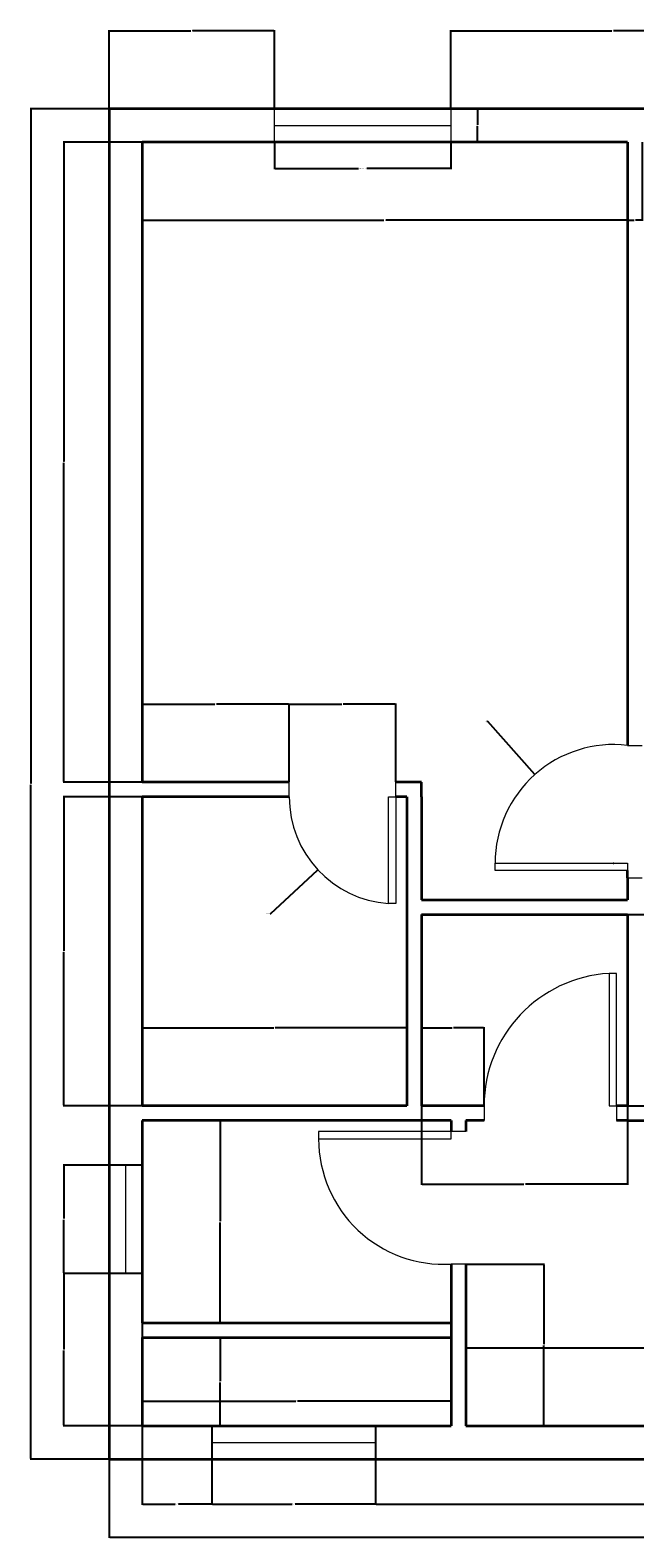
# Model space of a CAD drawing. Units: inches. Extents: x 2345 to 2781, y 2622 to 3032.
# Tile 1 of 3: x 2345 to 2509, y 2622 to 3032. Entities that reach past the tile are written whole.
import ezdxf

# ---------------------------------------------------------------- set-up
doc = ezdxf.new("R2010")
doc.units = ezdxf.units.IN
for name, color, linetype, lineweight in [('A-ANNO-DIMS', 2, 'Continuous', 18), ('A-DOOR', 3, 'Continuous', 18), ('A-GLAZ', 4, 'Continuous', 18), ('A-WALL', 7, 'Continuous', 35)]:
    doc.layers.add(name, color=color, linetype=linetype, lineweight=lineweight)
doc.styles.get("Standard").update_dxf_attribs({"font": 'arial.ttf'})
doc.dimstyles.get("Standard").update_dxf_attribs({"dimtxt": 0.18, "dimasz": 0.18, "dimexe": 0.18, "dimexo": 0.0625, "dimgap": 0.09, "dimtad": 0, "dimtih": 1, "dimtoh": 1, "dimdec": 4, "dimzin": 0, "dimdsep": 46, "dimtxsty": 'Standard', "dimcen": 0.09, "dimadec": 0, "dimazin": 0, "dimtfac": 1, "dimtdec": 4, "dimtofl": 0, "dimtmove": 0, "dimatfit": 3, "dimfxl": 1, "dimtolj": 1, "dimtzin": 0, "dimarcsym": 0})

# ---------------------------------------------------------------- blocks, each defined once
blk = doc.blocks.new('DOOR-36IN-SWING-A')
for p, q in [((36, 40), (34, 40)), ((34, 40), (34, 4)), ((36, 4), (36, 40)), ((0, 4), (0, 0)), ((34, 4), (36, 4)), ((36, 4), (36, 0))]:
    blk.add_line(p, q)
blk.add_arc((36.06, 4), 36.06, 93.2732, 180)
blk = doc.blocks.new('DOOR-36IN-SWING-B')
for p, q in [((0, 40), (0, 36)), ((36, 40), (36, 36)), ((0, 36), (0, 0)), ((2, 36), (0, 36)), ((2, 0), (2, 36)), ((0, 0), (2, 0))]:
    blk.add_line(p, q)
blk.add_arc((2, 34.06), 34.06, 270, 3.2732)
blk = doc.blocks.new('WIN-48IN')
for p, q in [((0, 0), (0, 9)), ((48, 0), (48, 9)), ((0, 4.5), (48, 4.5))]:
    blk.add_line(p, q)
blk = doc.blocks.new('*D8')
at = {"layer": 'A-ANNO-DIMS', "color": 0, "lineweight": -2, "transparency": 16777216}
for p, q in [((2411.27, 3001.74), (2411.27, 2994.42)), ((2459.27, 3001.74), (2459.27, 2994.42)), ((2411.45, 2994.6), (2434.15, 2994.6)), ((2459.09, 2994.6), (2436.39, 2994.6))]:
    blk.add_line(p, q, dxfattribs=at)
at = {"layer": 'A-ANNO-DIMS', "color": 0, "transparency": 16777216}
for points in [[(2411.45, 2994.63), (2411.45, 2994.57), (2411.27, 2994.6)], [(2459.09, 2994.63), (2459.09, 2994.57), (2459.27, 2994.6)]]:
    blk.add_solid(points, dxfattribs=at)
at = {"layer": 'Defpoints', "color": 0, "transparency": 16777216}
for p in [(2411.27, 3001.8), (2459.27, 3001.8), (2459.27, 2994.6)]:
    blk.add_point(p, dxfattribs=at)
at = {"layer": 'A-ANNO-DIMS', "color": 0, "transparency": 16777216, "insert": (2435.27, 2994.6), "char_height": 0.18, "attachment_point": 5}
blk.add_mtext('\\A1;WINDOW 48 TYP.', dxfattribs=at)
blk = doc.blocks.new('*D9')
at = {"layer": 'A-ANNO-DIMS', "color": 0, "lineweight": -2, "transparency": 16777216}
for p, q in [((2459.33, 3010.8), (2466.65, 3010.8)), ((2466.47, 3010.62), (2466.47, 3006.48)), ((2466.47, 3001.98), (2466.47, 3006.12)), ((2459.33, 3001.8), (2466.65, 3001.8))]:
    blk.add_line(p, q, dxfattribs=at)
at = {"layer": 'A-ANNO-DIMS', "color": 0, "transparency": 16777216}
for points in [[(2466.44, 3010.62), (2466.5, 3010.62), (2466.47, 3010.8)], [(2466.44, 3001.98), (2466.5, 3001.98), (2466.47, 3001.8)]]:
    blk.add_solid(points, dxfattribs=at)
at = {"layer": 'Defpoints', "color": 0, "transparency": 16777216}
for p in [(2459.27, 3010.8), (2466.47, 3010.8), (2459.27, 3001.8)]:
    blk.add_point(p, dxfattribs=at)
at = {"layer": 'A-ANNO-DIMS', "color": 0, "transparency": 16777216, "insert": (2466.47, 3006.3), "char_height": 0.18, "attachment_point": 5}
blk.add_mtext('\\A1;9 TYP.', dxfattribs=at)
blk = doc.blocks.new('*D10')
at = {"layer": 'A-ANNO-DIMS', "color": 0, "lineweight": -2, "transparency": 16777216}
for p, q in [((2366.27, 2643.74), (2366.27, 2622.37)), ((2768.27, 2643.74), (2768.27, 2622.37)), ((2366.45, 2622.55), (2566.98, 2622.55)), ((2768.09, 2622.55), (2567.56, 2622.55))]:
    blk.add_line(p, q, dxfattribs=at)
at = {"layer": 'A-ANNO-DIMS', "color": 0, "transparency": 16777216}
for points in [[(2366.45, 2622.58), (2366.45, 2622.52), (2366.27, 2622.55)], [(2768.09, 2622.58), (2768.09, 2622.52), (2768.27, 2622.55)]]:
    blk.add_solid(points, dxfattribs=at)
at = {"layer": 'Defpoints', "color": 0, "transparency": 16777216}
for p in [(2366.27, 2643.8), (2768.27, 2643.8), (2768.27, 2622.55)]:
    blk.add_point(p, dxfattribs=at)
at = {"layer": 'A-ANNO-DIMS', "color": 0, "transparency": 16777216, "insert": (2567.27, 2622.55), "char_height": 0.18, "attachment_point": 5}
blk.add_mtext('\\A1;402', dxfattribs=at)
blk = doc.blocks.new('*D11')
at = {"layer": 'A-ANNO-DIMS', "color": 0, "lineweight": -2, "transparency": 16777216}
for p, q in [((2366.21, 3010.8), (2344.84, 3010.8)), ((2345.02, 3010.62), (2345.02, 2827.48)), ((2345.02, 2643.98), (2345.02, 2827.12)), ((2366.21, 2643.8), (2344.84, 2643.8))]:
    blk.add_line(p, q, dxfattribs=at)
at = {"layer": 'A-ANNO-DIMS', "color": 0, "transparency": 16777216}
for points in [[(2344.99, 3010.62), (2345.05, 3010.62), (2345.02, 3010.8)], [(2344.99, 2643.98), (2345.05, 2643.98), (2345.02, 2643.8)]]:
    blk.add_solid(points, dxfattribs=at)
at = {"layer": 'Defpoints', "color": 0, "transparency": 16777216}
for p in [(2345.02, 3010.8), (2366.27, 3010.8), (2366.27, 2643.8)]:
    blk.add_point(p, dxfattribs=at)
at = {"layer": 'A-ANNO-DIMS', "color": 0, "transparency": 16777216, "insert": (2345.02, 2827.3), "char_height": 0.18, "attachment_point": 5}
blk.add_mtext('\\A1;367', dxfattribs=at)
blk = doc.blocks.new('*D12')
at = {"layer": 'A-ANNO-DIMS', "color": 0, "lineweight": -2, "transparency": 16777216}
for p, q in [((2366.27, 3010.87), (2366.27, 3032.23)), ((2366.45, 3032.05), (2388.55, 3032.05)), ((2411.09, 3032.05), (2389, 3032.05)), ((2411.27, 3010.87), (2411.27, 3032.23))]:
    blk.add_line(p, q, dxfattribs=at)
at = {"layer": 'A-ANNO-DIMS', "color": 0, "transparency": 16777216}
for points in [[(2366.45, 3032.08), (2366.45, 3032.02), (2366.27, 3032.05)], [(2411.09, 3032.08), (2411.09, 3032.02), (2411.27, 3032.05)]]:
    blk.add_solid(points, dxfattribs=at)
at = {"layer": 'Defpoints', "color": 0, "transparency": 16777216}
for p in [(2411.27, 3032.05), (2366.27, 3010.8), (2411.27, 3010.8)]:
    blk.add_point(p, dxfattribs=at)
at = {"layer": 'A-ANNO-DIMS', "color": 0, "transparency": 16777216, "insert": (2388.77, 3032.05), "char_height": 0.18, "attachment_point": 5}
blk.add_mtext('\\A1;45', dxfattribs=at)
blk = doc.blocks.new('*D13')
at = {"layer": 'A-ANNO-DIMS', "color": 0, "lineweight": -2, "transparency": 16777216}
for p, q in [((2459.27, 3010.87), (2459.27, 3032.23)), ((2459.45, 3032.05), (2503.05, 3032.05)), ((2547.09, 3032.05), (2503.49, 3032.05)), ((2547.27, 3010.87), (2547.27, 3032.23))]:
    blk.add_line(p, q, dxfattribs=at)
at = {"layer": 'A-ANNO-DIMS', "color": 0, "transparency": 16777216}
for points in [[(2459.45, 3032.08), (2459.45, 3032.02), (2459.27, 3032.05)], [(2547.09, 3032.08), (2547.09, 3032.02), (2547.27, 3032.05)]]:
    blk.add_solid(points, dxfattribs=at)
at = {"layer": 'Defpoints', "color": 0, "transparency": 16777216}
for p in [(2547.27, 3032.05), (2459.27, 3010.8), (2547.27, 3010.8)]:
    blk.add_point(p, dxfattribs=at)
at = {"layer": 'A-ANNO-DIMS', "color": 0, "transparency": 16777216, "insert": (2503.27, 3032.05), "char_height": 0.18, "attachment_point": 5}
blk.add_mtext('\\A1;88', dxfattribs=at)
blk = doc.blocks.new('*D15')
at = {"layer": 'A-ANNO-DIMS', "color": 0, "lineweight": -2, "transparency": 16777216}
for p, q in [((2375.27, 3001.74), (2375.27, 2980.37)), ((2507.27, 3001.74), (2507.27, 2980.37)), ((2375.45, 2980.55), (2440.99, 2980.55)), ((2507.09, 2980.55), (2441.55, 2980.55))]:
    blk.add_line(p, q, dxfattribs=at)
at = {"layer": 'A-ANNO-DIMS', "color": 0, "transparency": 16777216}
for points in [[(2375.45, 2980.58), (2375.45, 2980.52), (2375.27, 2980.55)], [(2507.09, 2980.58), (2507.09, 2980.52), (2507.27, 2980.55)]]:
    blk.add_solid(points, dxfattribs=at)
at = {"layer": 'Defpoints', "color": 0, "transparency": 16777216}
for p in [(2375.27, 3001.8), (2507.27, 3001.8), (2375.27, 2980.55)]:
    blk.add_point(p, dxfattribs=at)
at = {"layer": 'A-ANNO-DIMS', "color": 0, "transparency": 16777216, "insert": (2441.27, 2980.55), "char_height": 0.18, "attachment_point": 5}
blk.add_mtext('\\A1;132', dxfattribs=at)
blk = doc.blocks.new('*D16')
at = {"layer": 'A-ANNO-DIMS', "color": 0, "lineweight": -2, "transparency": 16777216}
for p, q in [((2507.27, 3001.74), (2507.27, 2980.37)), ((2511.27, 3001.74), (2511.27, 2980.37)), ((2507.45, 2980.55), (2509.12, 2980.55)), ((2511.09, 2980.55), (2509.42, 2980.55))]:
    blk.add_line(p, q, dxfattribs=at)
at = {"layer": 'A-ANNO-DIMS', "color": 0, "transparency": 16777216}
for points in [[(2507.45, 2980.58), (2507.45, 2980.52), (2507.27, 2980.55)], [(2511.09, 2980.58), (2511.09, 2980.52), (2511.27, 2980.55)]]:
    blk.add_solid(points, dxfattribs=at)
at = {"layer": 'Defpoints', "color": 0, "transparency": 16777216}
for p in [(2507.27, 3001.8), (2511.27, 3001.8), (2507.27, 2980.55)]:
    blk.add_point(p, dxfattribs=at)
at = {"layer": 'A-ANNO-DIMS', "color": 0, "transparency": 16777216, "insert": (2509.27, 2980.55), "char_height": 0.18, "attachment_point": 5}
blk.add_mtext('\\A1;4', dxfattribs=at)
blk = doc.blocks.new('*D24')
at = {"layer": 'A-ANNO-DIMS', "color": 0, "lineweight": -2, "transparency": 16777216}
for p, q in [((2375.21, 3001.8), (2353.84, 3001.8)), ((2354.02, 3001.62), (2354.02, 2914.98)), ((2354.02, 2827.98), (2354.02, 2914.62)), ((2375.21, 2827.8), (2353.84, 2827.8))]:
    blk.add_line(p, q, dxfattribs=at)
at = {"layer": 'A-ANNO-DIMS', "color": 0, "transparency": 16777216}
for points in [[(2353.99, 3001.62), (2354.05, 3001.62), (2354.02, 3001.8)], [(2353.99, 2827.98), (2354.05, 2827.98), (2354.02, 2827.8)]]:
    blk.add_solid(points, dxfattribs=at)
at = {"layer": 'Defpoints', "color": 0, "transparency": 16777216}
for p in [(2354.02, 3001.8), (2375.27, 3001.8), (2375.27, 2827.8)]:
    blk.add_point(p, dxfattribs=at)
at = {"layer": 'A-ANNO-DIMS', "color": 0, "transparency": 16777216, "insert": (2354.02, 2914.8), "char_height": 0.18, "attachment_point": 5}
blk.add_mtext('\\A1;174', dxfattribs=at)
blk = doc.blocks.new('*D26')
at = {"layer": 'A-ANNO-DIMS', "color": 0, "lineweight": -2, "transparency": 16777216}
for p, q in [((2375.27, 2827.87), (2375.27, 2849.23)), ((2375.45, 2849.05), (2395.05, 2849.05)), ((2415.09, 2849.05), (2395.49, 2849.05)), ((2415.27, 2827.87), (2415.27, 2849.23))]:
    blk.add_line(p, q, dxfattribs=at)
at = {"layer": 'A-ANNO-DIMS', "color": 0, "transparency": 16777216}
for points in [[(2375.45, 2849.08), (2375.45, 2849.02), (2375.27, 2849.05)], [(2415.09, 2849.08), (2415.09, 2849.02), (2415.27, 2849.05)]]:
    blk.add_solid(points, dxfattribs=at)
at = {"layer": 'Defpoints', "color": 0, "transparency": 16777216}
for p in [(2415.27, 2849.05), (2375.27, 2827.8), (2415.27, 2827.8)]:
    blk.add_point(p, dxfattribs=at)
at = {"layer": 'A-ANNO-DIMS', "color": 0, "transparency": 16777216, "insert": (2395.27, 2849.05), "char_height": 0.18, "attachment_point": 5}
blk.add_mtext('\\A1;40', dxfattribs=at)
blk = doc.blocks.new('*D27')
at = {"layer": 'A-ANNO-DIMS', "color": 0, "lineweight": -2, "transparency": 16777216}
for p, q in [((2415.27, 2827.87), (2415.27, 2849.23)), ((2415.45, 2849.05), (2429.55, 2849.05)), ((2444.09, 2849.05), (2429.99, 2849.05)), ((2444.27, 2827.87), (2444.27, 2849.23))]:
    blk.add_line(p, q, dxfattribs=at)
at = {"layer": 'A-ANNO-DIMS', "color": 0, "transparency": 16777216}
for points in [[(2415.45, 2849.08), (2415.45, 2849.02), (2415.27, 2849.05)], [(2444.09, 2849.08), (2444.09, 2849.02), (2444.27, 2849.05)]]:
    blk.add_solid(points, dxfattribs=at)
at = {"layer": 'Defpoints', "color": 0, "transparency": 16777216}
for p in [(2444.27, 2849.05), (2415.27, 2827.8), (2444.27, 2827.8)]:
    blk.add_point(p, dxfattribs=at)
at = {"layer": 'A-ANNO-DIMS', "color": 0, "transparency": 16777216, "insert": (2429.77, 2849.05), "char_height": 0.18, "attachment_point": 5}
blk.add_mtext('\\A1;29', dxfattribs=at)
blk = doc.blocks.new('*D32')
at = {"layer": 'A-ANNO-DIMS', "color": 0, "lineweight": -2, "transparency": 16777216}
for p, q in [((2375.27, 2739.87), (2375.27, 2761.23)), ((2375.45, 2761.05), (2411.05, 2761.05)), ((2447.09, 2761.05), (2411.49, 2761.05)), ((2447.27, 2739.87), (2447.27, 2761.23))]:
    blk.add_line(p, q, dxfattribs=at)
at = {"layer": 'A-ANNO-DIMS', "color": 0, "transparency": 16777216}
for points in [[(2375.45, 2761.08), (2375.45, 2761.02), (2375.27, 2761.05)], [(2447.09, 2761.08), (2447.09, 2761.02), (2447.27, 2761.05)]]:
    blk.add_solid(points, dxfattribs=at)
at = {"layer": 'Defpoints', "color": 0, "transparency": 16777216}
for p in [(2447.27, 2761.05), (2375.27, 2739.8), (2447.27, 2739.8)]:
    blk.add_point(p, dxfattribs=at)
at = {"layer": 'A-ANNO-DIMS', "color": 0, "transparency": 16777216, "insert": (2411.27, 2761.05), "char_height": 0.18, "attachment_point": 5}
blk.add_mtext('\\A1;72', dxfattribs=at)
blk = doc.blocks.new('*D33')
at = {"layer": 'A-ANNO-DIMS', "color": 0, "lineweight": -2, "transparency": 16777216}
for p, q in [((2375.21, 2823.8), (2353.84, 2823.8)), ((2354.02, 2823.62), (2354.02, 2781.98)), ((2354.02, 2739.98), (2354.02, 2781.62)), ((2375.21, 2739.8), (2353.84, 2739.8))]:
    blk.add_line(p, q, dxfattribs=at)
at = {"layer": 'A-ANNO-DIMS', "color": 0, "transparency": 16777216}
for points in [[(2353.99, 2823.62), (2354.05, 2823.62), (2354.02, 2823.8)], [(2353.99, 2739.98), (2354.05, 2739.98), (2354.02, 2739.8)]]:
    blk.add_solid(points, dxfattribs=at)
at = {"layer": 'Defpoints', "color": 0, "transparency": 16777216}
for p in [(2354.02, 2823.8), (2375.27, 2823.8), (2375.27, 2739.8)]:
    blk.add_point(p, dxfattribs=at)
at = {"layer": 'A-ANNO-DIMS', "color": 0, "transparency": 16777216, "insert": (2354.02, 2781.8), "char_height": 0.18, "attachment_point": 5}
blk.add_mtext('\\A1;84', dxfattribs=at)
blk = doc.blocks.new('*D34')
at = {"layer": 'A-ANNO-DIMS', "color": 0, "lineweight": -2, "transparency": 16777216}
for p, q in [((2507.33, 2791.8), (2528.7, 2791.8)), ((2528.52, 2791.62), (2528.52, 2765.98)), ((2528.52, 2739.98), (2528.52, 2765.62)), ((2507.33, 2739.8), (2528.7, 2739.8))]:
    blk.add_line(p, q, dxfattribs=at)
at = {"layer": 'A-ANNO-DIMS', "color": 0, "transparency": 16777216}
for points in [[(2528.49, 2791.62), (2528.55, 2791.62), (2528.52, 2791.8)], [(2528.49, 2739.98), (2528.55, 2739.98), (2528.52, 2739.8)]]:
    blk.add_solid(points, dxfattribs=at)
at = {"layer": 'Defpoints', "color": 0, "transparency": 16777216}
for p in [(2507.27, 2791.8), (2507.27, 2739.8), (2528.52, 2739.8)]:
    blk.add_point(p, dxfattribs=at)
at = {"layer": 'A-ANNO-DIMS', "color": 0, "transparency": 16777216, "insert": (2528.52, 2765.8), "char_height": 0.18, "attachment_point": 5}
blk.add_mtext('\\A1;52', dxfattribs=at)
blk = doc.blocks.new('*D35')
at = {"layer": 'A-ANNO-DIMS', "color": 0, "lineweight": -2, "transparency": 16777216}
for p, q in [((2451.27, 2739.74), (2451.27, 2718.37)), ((2507.27, 2739.74), (2507.27, 2718.37)), ((2451.45, 2718.55), (2479.05, 2718.55)), ((2507.09, 2718.55), (2479.49, 2718.55))]:
    blk.add_line(p, q, dxfattribs=at)
at = {"layer": 'A-ANNO-DIMS', "color": 0, "transparency": 16777216}
for points in [[(2451.45, 2718.58), (2451.45, 2718.52), (2451.27, 2718.55)], [(2507.09, 2718.58), (2507.09, 2718.52), (2507.27, 2718.55)]]:
    blk.add_solid(points, dxfattribs=at)
at = {"layer": 'Defpoints', "color": 0, "transparency": 16777216}
for p in [(2451.27, 2739.8), (2507.27, 2739.8), (2451.27, 2718.55)]:
    blk.add_point(p, dxfattribs=at)
at = {"layer": 'A-ANNO-DIMS', "color": 0, "transparency": 16777216, "insert": (2479.27, 2718.55), "char_height": 0.18, "attachment_point": 5}
blk.add_mtext('\\A1;56', dxfattribs=at)
blk = doc.blocks.new('*D37')
at = {"layer": 'A-ANNO-DIMS', "color": 0, "lineweight": -2, "transparency": 16777216}
for p, q in [((2451.27, 2739.87), (2451.27, 2761.23)), ((2451.45, 2761.05), (2459.56, 2761.05)), ((2468.09, 2761.05), (2459.98, 2761.05)), ((2468.27, 2739.87), (2468.27, 2761.23))]:
    blk.add_line(p, q, dxfattribs=at)
at = {"layer": 'A-ANNO-DIMS', "color": 0, "transparency": 16777216}
for points in [[(2451.45, 2761.08), (2451.45, 2761.02), (2451.27, 2761.05)], [(2468.09, 2761.08), (2468.09, 2761.02), (2468.27, 2761.05)]]:
    blk.add_solid(points, dxfattribs=at)
at = {"layer": 'Defpoints', "color": 0, "transparency": 16777216}
for p in [(2468.27, 2761.05), (2451.27, 2739.8), (2468.27, 2739.8)]:
    blk.add_point(p, dxfattribs=at)
at = {"layer": 'A-ANNO-DIMS', "color": 0, "transparency": 16777216, "insert": (2459.77, 2761.05), "char_height": 0.18, "attachment_point": 5}
blk.add_mtext('\\A1;17', dxfattribs=at)
blk = doc.blocks.new('*D49')
at = {"layer": 'A-ANNO-DIMS', "color": 0, "lineweight": -2, "transparency": 16777216}
for p, q in [((2375.27, 2680.74), (2375.27, 2659.37)), ((2459.27, 2680.74), (2459.27, 2659.37)), ((2375.45, 2659.55), (2417.05, 2659.55)), ((2459.09, 2659.55), (2417.49, 2659.55))]:
    blk.add_line(p, q, dxfattribs=at)
at = {"layer": 'A-ANNO-DIMS', "color": 0, "transparency": 16777216}
for points in [[(2375.45, 2659.58), (2375.45, 2659.52), (2375.27, 2659.55)], [(2459.09, 2659.58), (2459.09, 2659.52), (2459.27, 2659.55)]]:
    blk.add_solid(points, dxfattribs=at)
at = {"layer": 'Defpoints', "color": 0, "transparency": 16777216}
for p in [(2375.27, 2680.8), (2459.27, 2680.8), (2375.27, 2659.55)]:
    blk.add_point(p, dxfattribs=at)
at = {"layer": 'A-ANNO-DIMS', "color": 0, "transparency": 16777216, "insert": (2417.27, 2659.55), "char_height": 0.18, "attachment_point": 5}
blk.add_mtext('\\A1;84', dxfattribs=at)
blk = doc.blocks.new('*D50')
at = {"layer": 'A-ANNO-DIMS', "color": 0, "lineweight": -2, "transparency": 16777216}
for p, q in [((2375.33, 2676.8), (2396.7, 2676.8)), ((2396.52, 2676.62), (2396.52, 2664.98)), ((2396.52, 2652.98), (2396.52, 2664.62)), ((2375.33, 2652.8), (2396.7, 2652.8))]:
    blk.add_line(p, q, dxfattribs=at)
at = {"layer": 'A-ANNO-DIMS', "color": 0, "transparency": 16777216}
for points in [[(2396.49, 2676.62), (2396.55, 2676.62), (2396.52, 2676.8)], [(2396.49, 2652.98), (2396.55, 2652.98), (2396.52, 2652.8)]]:
    blk.add_solid(points, dxfattribs=at)
at = {"layer": 'Defpoints', "color": 0, "transparency": 16777216}
for p in [(2375.27, 2676.8), (2375.27, 2652.8), (2396.52, 2652.8)]:
    blk.add_point(p, dxfattribs=at)
at = {"layer": 'A-ANNO-DIMS', "color": 0, "transparency": 16777216, "insert": (2396.52, 2664.8), "char_height": 0.18, "attachment_point": 5}
blk.add_mtext('\\A1;24', dxfattribs=at)
blk = doc.blocks.new('*D51')
at = {"layer": 'A-ANNO-DIMS', "color": 0, "lineweight": -2, "transparency": 16777216}
for p, q in [((2375.33, 2735.8), (2396.7, 2735.8)), ((2396.52, 2735.62), (2396.52, 2708.48)), ((2396.52, 2680.98), (2396.52, 2708.12)), ((2375.33, 2680.8), (2396.7, 2680.8))]:
    blk.add_line(p, q, dxfattribs=at)
at = {"layer": 'A-ANNO-DIMS', "color": 0, "transparency": 16777216}
for points in [[(2396.49, 2735.62), (2396.55, 2735.62), (2396.52, 2735.8)], [(2396.49, 2680.98), (2396.55, 2680.98), (2396.52, 2680.8)]]:
    blk.add_solid(points, dxfattribs=at)
at = {"layer": 'Defpoints', "color": 0, "transparency": 16777216}
for p in [(2375.27, 2735.8), (2375.27, 2680.8), (2396.52, 2680.8)]:
    blk.add_point(p, dxfattribs=at)
at = {"layer": 'A-ANNO-DIMS', "color": 0, "transparency": 16777216, "insert": (2396.52, 2708.3), "char_height": 0.18, "attachment_point": 5}
blk.add_mtext('\\A1;55', dxfattribs=at)
blk = doc.blocks.new('*D52')
at = {"layer": 'A-ANNO-DIMS', "color": 0, "lineweight": -2, "transparency": 16777216}
for p, q in [((2463.27, 2652.87), (2463.27, 2674.23)), ((2463.45, 2674.05), (2537.99, 2674.05)), ((2613.09, 2674.05), (2538.55, 2674.05)), ((2613.27, 2652.87), (2613.27, 2674.23))]:
    blk.add_line(p, q, dxfattribs=at)
at = {"layer": 'A-ANNO-DIMS', "color": 0, "transparency": 16777216}
for points in [[(2463.45, 2674.08), (2463.45, 2674.02), (2463.27, 2674.05)], [(2613.09, 2674.08), (2613.09, 2674.02), (2613.27, 2674.05)]]:
    blk.add_solid(points, dxfattribs=at)
at = {"layer": 'Defpoints', "color": 0, "transparency": 16777216}
for p in [(2613.27, 2674.05), (2463.27, 2652.8), (2613.27, 2652.8)]:
    blk.add_point(p, dxfattribs=at)
at = {"layer": 'A-ANNO-DIMS', "color": 0, "transparency": 16777216, "insert": (2538.27, 2674.05), "char_height": 0.18, "attachment_point": 5}
blk.add_mtext('\\A1;150', dxfattribs=at)
blk = doc.blocks.new('*D55')
at = {"layer": 'A-ANNO-DIMS', "color": 0, "lineweight": -2, "transparency": 16777216}
for p, q in [((2463.334411, 2696.80295), (2484.701911, 2696.80295)), ((2484.521911, 2696.62295), (2484.521911, 2674.98295)), ((2484.521911, 2652.98295), (2484.521911, 2674.62295)), ((2463.334411, 2652.80295), (2484.701911, 2652.80295))]:
    blk.add_line(p, q, dxfattribs=at)
at = {"layer": 'A-ANNO-DIMS', "color": 0, "transparency": 16777216}
for points in [[(2484.491911, 2696.62295), (2484.551911, 2696.62295), (2484.521911, 2696.80295)], [(2484.491911, 2652.98295), (2484.551911, 2652.98295), (2484.521911, 2652.80295)]]:
    blk.add_solid(points, dxfattribs=at)
at = {"layer": 'Defpoints', "color": 0, "transparency": 16777216}
for p in [(2463.271911, 2696.80295), (2463.271911, 2652.80295), (2484.521911, 2652.80295)]:
    blk.add_point(p, dxfattribs=at)
at = {"layer": 'A-ANNO-DIMS', "color": 0, "transparency": 16777216, "insert": (2484.521911, 2674.80295), "char_height": 0.18, "attachment_point": 5}
blk.add_mtext('\\A1;44', dxfattribs=at)
blk = doc.blocks.new('*D57')
at = {"layer": 'A-ANNO-DIMS', "color": 0, "lineweight": -2, "transparency": 16777216}
for p, q in [((2375.27, 2652.74), (2375.27, 2631.37)), ((2394.21, 2652.74), (2394.21, 2631.37)), ((2375.45, 2631.55), (2384.28, 2631.55)), ((2394.03, 2631.55), (2385.19, 2631.55))]:
    blk.add_line(p, q, dxfattribs=at)
at = {"layer": 'A-ANNO-DIMS', "color": 0, "transparency": 16777216}
for points in [[(2375.45, 2631.58), (2375.45, 2631.52), (2375.27, 2631.55)], [(2394.03, 2631.58), (2394.03, 2631.52), (2394.21, 2631.55)]]:
    blk.add_solid(points, dxfattribs=at)
at = {"layer": 'Defpoints', "color": 0, "transparency": 16777216}
for p in [(2375.27, 2652.8), (2394.21, 2652.8), (2375.27, 2631.55)]:
    blk.add_point(p, dxfattribs=at)
at = {"layer": 'A-ANNO-DIMS', "color": 0, "transparency": 16777216, "insert": (2384.74, 2631.55), "char_height": 0.18, "attachment_point": 5}
blk.add_mtext('\\A1;18.934', dxfattribs=at)
blk = doc.blocks.new('*D58')
at = {"layer": 'A-ANNO-DIMS', "color": 0, "lineweight": -2, "transparency": 16777216}
for p, q in [((2394.21, 2652.74), (2394.21, 2631.37)), ((2438.77, 2652.74), (2438.77, 2631.37)), ((2394.39, 2631.55), (2416.09, 2631.55)), ((2438.59, 2631.55), (2416.88, 2631.55))]:
    blk.add_line(p, q, dxfattribs=at)
at = {"layer": 'A-ANNO-DIMS', "color": 0, "transparency": 16777216}
for points in [[(2394.39, 2631.58), (2394.39, 2631.52), (2394.21, 2631.55)], [(2438.59, 2631.58), (2438.59, 2631.52), (2438.77, 2631.55)]]:
    blk.add_solid(points, dxfattribs=at)
at = {"layer": 'Defpoints', "color": 0, "transparency": 16777216}
for p in [(2394.21, 2652.8), (2438.77, 2652.8), (2394.21, 2631.55)]:
    blk.add_point(p, dxfattribs=at)
at = {"layer": 'A-ANNO-DIMS', "color": 0, "transparency": 16777216, "insert": (2416.49, 2631.55), "char_height": 0.18, "attachment_point": 5}
blk.add_mtext('\\A1;44.56', dxfattribs=at)
blk = doc.blocks.new('*D59')
at = {"layer": 'A-ANNO-DIMS', "color": 0, "lineweight": -2, "transparency": 16777216}
for p, q in [((2438.77, 2652.74), (2438.77, 2631.37)), ((2637.97, 2652.74), (2637.97, 2631.37)), ((2438.95, 2631.55), (2537.98, 2631.55)), ((2637.79, 2631.55), (2538.75, 2631.55))]:
    blk.add_line(p, q, dxfattribs=at)
at = {"layer": 'A-ANNO-DIMS', "color": 0, "transparency": 16777216}
for points in [[(2438.95, 2631.58), (2438.95, 2631.52), (2438.77, 2631.55)], [(2637.79, 2631.58), (2637.79, 2631.52), (2637.97, 2631.55)]]:
    blk.add_solid(points, dxfattribs=at)
at = {"layer": 'Defpoints', "color": 0, "transparency": 16777216}
for p in [(2438.77, 2652.8), (2637.97, 2652.8), (2438.77, 2631.55)]:
    blk.add_point(p, dxfattribs=at)
at = {"layer": 'A-ANNO-DIMS', "color": 0, "transparency": 16777216, "insert": (2538.37, 2631.55), "char_height": 0.18, "attachment_point": 5}
blk.add_mtext('\\A1;199.2', dxfattribs=at)
blk = doc.blocks.new('*D63')
at = {"layer": 'A-ANNO-DIMS', "color": 0, "lineweight": -2, "transparency": 16777216}
for p, q in [((2375.21, 2723.72), (2353.84, 2723.72)), ((2354.02, 2723.54), (2354.02, 2709.16)), ((2354.02, 2694.41), (2354.02, 2708.79)), ((2375.21, 2694.23), (2353.84, 2694.23))]:
    blk.add_line(p, q, dxfattribs=at)
at = {"layer": 'A-ANNO-DIMS', "color": 0, "transparency": 16777216}
for points in [[(2353.99, 2723.54), (2354.05, 2723.54), (2354.02, 2723.72)], [(2353.99, 2694.41), (2354.05, 2694.41), (2354.02, 2694.23)]]:
    blk.add_solid(points, dxfattribs=at)
at = {"layer": 'Defpoints', "color": 0, "transparency": 16777216}
for p in [(2354.02, 2723.72), (2375.27, 2723.72), (2375.27, 2694.23)]:
    blk.add_point(p, dxfattribs=at)
at = {"layer": 'A-ANNO-DIMS', "color": 0, "transparency": 16777216, "insert": (2354.02, 2708.97), "char_height": 0.18, "attachment_point": 5}
blk.add_mtext('\\A1;29.48', dxfattribs=at)
blk = doc.blocks.new('*D64')
at = {"layer": 'A-ANNO-DIMS', "color": 0, "lineweight": -2, "transparency": 16777216}
for p, q in [((2375.21, 2694.23), (2353.84, 2694.23)), ((2354.02, 2694.05), (2354.02, 2673.7)), ((2354.02, 2652.98), (2354.02, 2673.34)), ((2375.21, 2652.8), (2353.84, 2652.8))]:
    blk.add_line(p, q, dxfattribs=at)
at = {"layer": 'A-ANNO-DIMS', "color": 0, "transparency": 16777216}
for points in [[(2353.99, 2694.05), (2354.05, 2694.05), (2354.02, 2694.23)], [(2353.99, 2652.98), (2354.05, 2652.98), (2354.02, 2652.8)]]:
    blk.add_solid(points, dxfattribs=at)
at = {"layer": 'Defpoints', "color": 0, "transparency": 16777216}
for p in [(2354.02, 2694.23), (2375.27, 2694.23), (2375.27, 2652.8)]:
    blk.add_point(p, dxfattribs=at)
at = {"layer": 'A-ANNO-DIMS', "color": 0, "transparency": 16777216, "insert": (2354.02, 2673.52), "char_height": 0.18, "attachment_point": 5}
blk.add_mtext('\\A1;41.43', dxfattribs=at)
blk = doc.blocks.new('*D67')
at = {"layer": 'A-ANNO-DIMS', "color": 0, "lineweight": -2, "transparency": 16777216}
for p, q in [((2469.06, 2844.34), (2469.24, 2844.34)), ((2469.24, 2844.34), (2481.97, 2830.02)), ((2503.4, 2805.8), (2503.58, 2805.8)), ((2503.49, 2805.71), (2503.49, 2805.89))]:
    blk.add_line(p, q, dxfattribs=at)
at = {"layer": 'A-ANNO-DIMS', "color": 0, "transparency": 16777216}
blk.add_solid([(2481.99, 2830.04), (2481.94, 2830), (2482.09, 2829.89)], dxfattribs=at)
at = {"layer": 'Defpoints', "color": 0, "transparency": 16777216}
for p in [(2482.09, 2829.89), (2503.49, 2805.8)]:
    blk.add_point(p, dxfattribs=at)
at = {"layer": 'A-ANNO-DIMS', "color": 0, "transparency": 16777216, "insert": (2468.58, 2844.34), "char_height": 0.18, "attachment_point": 5}
blk.add_mtext('\\A1;R32.22', dxfattribs=at)
blk = doc.blocks.new('*D68')
at = {"layer": 'A-ANNO-DIMS', "color": 0, "lineweight": -2, "transparency": 16777216}
for p, q in [((2444.26, 2823.8), (2444.44, 2823.8)), ((2444.35, 2823.71), (2444.35, 2823.89)), ((2410.3, 2792.1), (2422.94, 2803.87)), ((2410.12, 2792.1), (2410.3, 2792.1))]:
    blk.add_line(p, q, dxfattribs=at)
at = {"layer": 'A-ANNO-DIMS', "color": 0, "transparency": 16777216}
blk.add_solid([(2422.91, 2803.89), (2422.96, 2803.85), (2423.07, 2803.99)], dxfattribs=at)
at = {"layer": 'Defpoints', "color": 0, "transparency": 16777216}
for p in [(2444.35, 2823.8), (2423.07, 2803.99)]:
    blk.add_point(p, dxfattribs=at)
at = {"layer": 'A-ANNO-DIMS', "color": 0, "transparency": 16777216, "insert": (2409.57, 2792.1), "char_height": 0.18, "attachment_point": 5}
blk.add_mtext('\\A1;R29.074', dxfattribs=at)

msp = doc.modelspace()

# ---------------------------------------------------------------- linework, layer by layer
at = {"layer": 'A-DOOR'}
for p, q in [((2507.2719, 2837.803), (2511.2719, 2837.803)), ((2415.2719, 2823.8029), (2415.2719, 2827.8029)), ((2444.2719, 2823.8029), (2444.2719, 2827.8029)), ((2442.2719, 2794.803), (2442.2719, 2823.8029)), ((2442.2719, 2823.8029), (2445.7719, 2823.8029)), ((2444.2719, 2823.8029), (2444.2719, 2794.803)), ((2471.2719, 2803.803), (2471.2719, 2805.8029)), ((2471.2719, 2805.8029), (2507.2719, 2805.8029)), ((2507.2719, 2803.803), (2471.2719, 2803.803)), ((2507.2719, 2805.8029), (2507.2719, 2803.803)), ((2507.2719, 2801.803), (2511.2719, 2801.803)), ((2444.2719, 2794.803), (2442.2719, 2794.803))]:
    msp.add_line(p, q, dxfattribs=at)
for centre, radius, start, end in [((2503.4941, 2805.8029), 32.2222, 83.267079, 180), ((2444.346, 2823.8029), 29.0741, 180, 265.909183)]:
    msp.add_arc(centre, radius, start, end, dxfattribs=at)
at = {"layer": 'A-GLAZ'}
for p, q in [((2375.2719, 2723.7151), (2366.2719, 2723.7151)), ((2370.7719, 2723.7151), (2370.7719, 2694.2347)), ((2375.2719, 2694.2347), (2366.2719, 2694.2347)), ((2394.2063, 2652.8029), (2394.2063, 2643.8029)), ((2438.7687, 2652.8029), (2438.7687, 2643.8029)), ((2394.2063, 2648.303), (2438.7687, 2648.303))]:
    msp.add_line(p, q, dxfattribs=at)
at = {"layer": 'A-WALL'}
for p, q in [((2768.2719, 3010.8029), (2366.2719, 3010.8029)), ((2366.2719, 3010.8029), (2366.2719, 2643.8029)), ((2375.2719, 3001.8029), (2375.2719, 2827.8029)), ((2507.2719, 3001.8029), (2375.2719, 3001.8029)), ((2507.2719, 3001.8029), (2507.2719, 2837.803)), ((2415.2719, 2827.8029), (2375.2719, 2827.8029)), ((2451.2719, 2827.8029), (2444.2719, 2827.8029)), ((2451.2719, 2823.8029), (2451.2719, 2827.8029)), ((2375.2719, 2823.8029), (2375.2719, 2739.8029)), ((2415.2719, 2823.8029), (2375.2719, 2823.8029)), ((2447.2719, 2823.8029), (2444.2719, 2823.8029)), ((2447.2719, 2823.8029), (2447.2719, 2739.8029)), ((2451.2719, 2823.8029), (2451.2719, 2795.803)), ((2451.2719, 2823.8029), (2451.2719, 2795.803)), ((2507.2719, 2801.803), (2507.2719, 2803.803)), ((2507.2719, 2801.803), (2507.2719, 2795.803)), ((2451.2719, 2795.803), (2507.2719, 2795.803)), ((2451.2719, 2791.8029), (2507.2719, 2791.8029)), ((2451.2719, 2791.8029), (2451.2719, 2779.803)), ((2451.2719, 2791.8029), (2451.2719, 2779.803)), ((2507.2719, 2791.8029), (2507.2719, 2779.803)), ((2451.2719, 2779.803), (2451.2719, 2775.0862)), ((2507.2719, 2779.803), (2507.2719, 2774.511)), ((2451.2719, 2775.803), (2451.2719, 2739.8029)), ((2451.2719, 2775.803), (2451.2719, 2739.8029)), ((2507.2719, 2775.803), (2507.2719, 2739.8029)), ((2447.2719, 2739.8029), (2375.2719, 2739.8029)), ((2468.2719, 2739.8029), (2451.2719, 2739.8029)), ((2507.2719, 2739.8029), (2504.2719, 2739.8029)), ((2375.2719, 2735.8029), (2375.2719, 2680.8029)), ((2459.2719, 2735.8029), (2375.2719, 2735.8029)), ((2459.2719, 2735.8029), (2459.2719, 2732.803)), ((2468.2719, 2735.8029), (2463.2719, 2735.8029)), ((2463.2719, 2735.8029), (2463.2719, 2732.803)), ((2507.2719, 2735.8029), (2504.2719, 2735.8029)), ((2507.2719, 2735.8029), (2511.7641, 2735.8029)), ((2459.2719, 2696.8029), (2459.2719, 2652.8029)), ((2463.2719, 2696.8029), (2463.2719, 2652.8029)), ((2375.2719, 2680.8029), (2459.2719, 2680.8029)), ((2375.2719, 2676.8029), (2459.2719, 2676.8029)), ((2375.2719, 2676.8029), (2375.2719, 2652.8029)), ((2375.2719, 2652.8029), (2459.2719, 2652.8029)), ((2463.2719, 2652.8029), (2507.2719, 2652.8029)), ((2507.2719, 2652.8029), (2513.846, 2652.8029)), ((2366.2719, 2643.8029), (2768.2719, 2643.8029))]:
    msp.add_line(p, q, dxfattribs=at)

# ---------------------------------------------------------------- block references
at = {"layer": 'A-DOOR'}
msp.add_blockref('DOOR-36IN-SWING-A', (2468.272, 2735.803), dxfattribs=at)
at = {"layer": 'A-DOOR', "rotation": 270.0000000000041}
msp.add_blockref('DOOR-36IN-SWING-B', (2423.272, 2732.8029), dxfattribs=at)
at = {"layer": 'A-GLAZ'}
msp.add_blockref('WIN-48IN', (2411.272, 3001.803), dxfattribs=at)

# ---------------------------------------------------------------- dimensions: what is measured, and where the dimension line sits
at = {"layer": 'A-ANNO-DIMS'}
for base, p1, p2, picture, middle in [((2411.2719, 3032.0529), (2366.2719, 3010.8029), (2411.2719, 3010.8029), '*D12', (2388.7719, 3032.0529)), ((2547.2719, 3032.0529), (2459.2719, 3010.8029), (2547.2719, 3010.8029), '*D13', (2503.2719, 3032.0529)), ((2415.2719, 2849.0529), (2375.2719, 2827.8029), (2415.2719, 2827.8029), '*D26', (2395.2719, 2849.0529)), ((2444.2719, 2849.0529), (2415.2719, 2827.8029), (2444.2719, 2827.8029), '*D27', (2429.7719, 2849.0529)), ((2447.2719, 2761.0529), (2375.2719, 2739.8029), (2447.2719, 2739.8029), '*D32', (2411.2719, 2761.0529)), ((2468.2719, 2761.0529), (2451.2719, 2739.8029), (2468.2719, 2739.8029), '*D37', (2459.7719, 2761.0529)), ((2768.2719, 2622.5529), (2366.2719, 2643.8029), (2768.2719, 2643.8029), '*D10', (2567.2719, 2622.5529))]:
    dim = msp.add_linear_dim(base=base, p1=p1, p2=p2, dimstyle='Standard', override={"dimdec": 0, "dimlfac": 1, "dimrnd": 0, "dimzin": 0, "dimdsep": 46, "dimlunit": 2}, dxfattribs=at)
    dim.commit()
    dim.dimension.update_dxf_attribs({"geometry": picture, "text_midpoint": middle})
for base, p1, p2, angle, override, picture, middle in [((2345.0219, 3010.8029), (2366.2719, 2643.8029), (2366.2719, 3010.8029), 90, {"dimdec": 0, "dimlfac": 1, "dimrnd": 0, "dimzin": 0, "dimdsep": 46, "dimlunit": 2}, '*D11', (2345.0219, 2827.3029)), ((2354.0219, 3001.8029), (2375.2719, 2827.8029), (2375.2719, 3001.8029), 90, {"dimdec": 0, "dimlfac": 1, "dimrnd": 0, "dimzin": 0, "dimdsep": 46, "dimlunit": 2}, '*D24', (2354.0219, 2914.8029)), ((2375.2719, 2980.5529), (2507.2719, 3001.8029), (2375.2719, 3001.8029), 180, {"dimdec": 0, "dimlfac": 1, "dimrnd": 0, "dimzin": 0, "dimdsep": 46, "dimlunit": 2}, '*D15', (2441.2719, 2980.5529)), ((2507.2719, 2980.5529), (2511.2719, 3001.8029), (2507.2719, 3001.8029), 180, {"dimdec": 0, "dimlfac": 1, "dimrnd": 0, "dimzin": 0, "dimdsep": 46, "dimlunit": 2}, '*D16', (2509.2719, 2980.5529)), ((2354.0219, 2823.8029), (2375.2719, 2739.8029), (2375.2719, 2823.8029), 90, {"dimdec": 0, "dimlfac": 1, "dimrnd": 0, "dimzin": 0, "dimdsep": 46, "dimlunit": 2}, '*D33', (2354.0219, 2781.8029)), ((2528.5219, 2739.8029), (2507.2719, 2791.8029), (2507.2719, 2739.8029), 270, {"dimdec": 0, "dimlfac": 1, "dimrnd": 0, "dimzin": 0, "dimdsep": 46, "dimlunit": 2}, '*D34', (2528.5219, 2765.8029)), ((2451.2719, 2718.5529), (2507.2719, 2739.8029), (2451.2719, 2739.8029), 180, {"dimdec": 0, "dimlfac": 1, "dimrnd": 0, "dimzin": 0, "dimdsep": 46, "dimlunit": 2}, '*D35', (2479.2719, 2718.5529)), ((2396.5219, 2680.8029), (2375.2719, 2735.8029), (2375.2719, 2680.8029), 270, {"dimdec": 0, "dimlfac": 1, "dimrnd": 0, "dimzin": 0, "dimdsep": 46, "dimlunit": 2}, '*D51', (2396.5219, 2708.3029)), ((2354.0219, 2723.7151), (2375.2719, 2694.2347), (2375.2719, 2723.7151), 90, {"dimdec": 2, "dimlfac": 1, "dimrnd": 0, "dimzin": 0, "dimdsep": 46, "dimlunit": 2}, '*D63', (2354.0219, 2708.9749)), ((2354.0219, 2694.2347), (2375.2719, 2652.8029), (2375.2719, 2694.2347), 90, {"dimdec": 2, "dimlfac": 1, "dimrnd": 0, "dimzin": 0, "dimdsep": 46, "dimlunit": 2}, '*D64', (2354.0219, 2673.5188)), ((2484.5219, 2652.8029), (2463.2719, 2696.8029), (2463.2719, 2652.8029), 270, {"dimdec": 0, "dimlfac": 1, "dimrnd": 0, "dimzin": 0, "dimdsep": 46, "dimlunit": 2}, '*D55', (2484.5219, 2674.8029)), ((2375.2719, 2659.5529), (2459.2719, 2680.8029), (2375.2719, 2680.8029), 180, {"dimdec": 0, "dimlfac": 1, "dimrnd": 0, "dimzin": 0, "dimdsep": 46, "dimlunit": 2}, '*D49', (2417.2719, 2659.5529)), ((2396.5219, 2652.8029), (2375.2719, 2676.8029), (2375.2719, 2652.8029), 270, {"dimdec": 0, "dimlfac": 1, "dimrnd": 0, "dimzin": 0, "dimdsep": 46, "dimlunit": 2}, '*D50', (2396.5219, 2664.8029)), ((2613.2719, 2674.0529), (2463.2719, 2652.8029), (2613.2719, 2652.8029), 0, {"dimdec": 0, "dimlfac": 1, "dimrnd": 0, "dimzin": 0, "dimdsep": 46, "dimlunit": 2}, '*D52', (2538.2719, 2674.0529)), ((2375.2719, 2631.5529), (2394.2063, 2652.8029), (2375.2719, 2652.8029), 180, {"dimdec": 3, "dimlfac": 1, "dimrnd": 0, "dimzin": 0, "dimdsep": 46, "dimlunit": 2}, '*D57', (2384.7391, 2631.5529)), ((2394.2063, 2631.5529), (2438.7687, 2652.8029), (2394.2063, 2652.8029), 180, {"dimdec": 2, "dimlfac": 1, "dimrnd": 0, "dimzin": 0, "dimdsep": 46, "dimlunit": 2}, '*D58', (2416.4875, 2631.5529)), ((2438.7687, 2631.5529), (2637.9676, 2652.8029), (2438.7687, 2652.8029), 180, {"dimdec": 1, "dimlfac": 1, "dimrnd": 0, "dimzin": 0, "dimdsep": 46, "dimlunit": 2}, '*D59', (2538.3681, 2631.5529))]:
    dim = msp.add_linear_dim(base=base, p1=p1, p2=p2, angle=angle, dimstyle='Standard', override=override, dxfattribs=at)
    dim.commit()
    dim.dimension.update_dxf_attribs({"geometry": picture, "text_midpoint": middle})
dim = msp.add_linear_dim(base=(2466.4719, 3010.8029), p1=(2459.2719, 3001.8029), p2=(2459.2719, 3010.8029), angle=90, text='<> TYP.', dimstyle='Standard', override={"dimdec": 0, "dimlfac": 1, "dimrnd": 0, "dimzin": 0, "dimdsep": 46, "dimlunit": 2}, dxfattribs=at)
dim.commit()
dim.dimension.update_dxf_attribs({"geometry": '*D9', "text_midpoint": (2466.4719, 3006.303)})
dim = msp.add_linear_dim(base=(2459.2719, 2994.603), p1=(2411.2719, 3001.8029), p2=(2459.2719, 3001.8029), text='WINDOW <> TYP.', dimstyle='Standard', override={"dimdec": 0, "dimlfac": 1, "dimrnd": 0, "dimzin": 0, "dimdsep": 46, "dimlunit": 2}, dxfattribs=at)
dim.commit()
dim.dimension.update_dxf_attribs({"geometry": '*D8', "text_midpoint": (2435.2719, 2994.603)})
for center, mpoint, override, picture, middle in [((2503.4941, 2805.8029), (2482.0869, 2829.8861), {"dimdec": 2, "dimlfac": 1, "dimrnd": 0, "dimzin": 0, "dimdsep": 46, "dimlunit": 2}, '*D67', (2468.5836, 2844.3361)), ((2444.346, 2823.8029), (2423.0671, 2803.9911), {"dimdec": 3, "dimlfac": 1, "dimrnd": 0, "dimzin": 0, "dimdsep": 46, "dimlunit": 2}, '*D68', (2409.5704, 2792.104))]:
    dim = msp.add_radius_dim(center=center, mpoint=mpoint, dimstyle='Standard', override=override, dxfattribs=at)
    dim.commit()
    dim.dimension.update_dxf_attribs({"geometry": picture, "text_midpoint": middle, "dimtype": 164})

doc.saveas('drawing.dxf')
